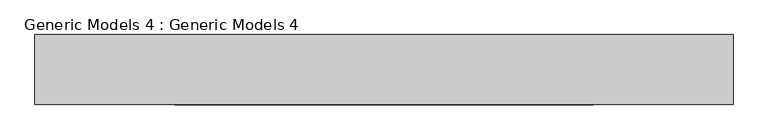
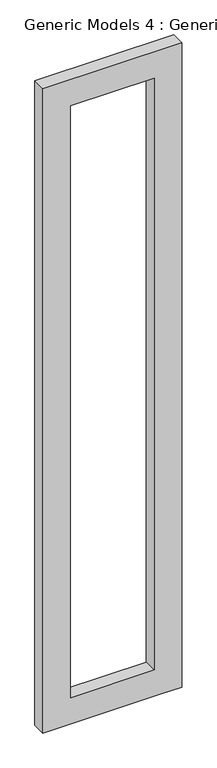
"""IFC4 building model written with IfcOpenShell, lengths in millimetres: proxy geometry, Generic Models 4 : Generic Models 4."""

from ifc_helpers import new_model, si_unit, frame, origin, place, context, project, spatial, polyline, outline, extrude, source, transform, mapped, element, save


def generic_models_4_generic_models_4_a39c55b3(model_context):
    return source(origin(), model_context, "Body", "SweptSolid", [
        extrude(outline(polyline([(7467.6, -14902.5371373), (7467.6, -16426.5371373), (0.0, -16426.5371373), (0.0, -15131.1371373), (0.0, -14902.5371373), (6426.2, -14902.5371373), (7467.6, -14902.5371373)]), holes=[polyline([(304.8, -16121.7371373), (7162.8, -16121.7371373), (7162.8, -15207.3371373), (304.8, -15207.3371373), (304.8, -16121.7371373)])]), frame((0.0, -3532.661407, 0.0), z_axis=(0.0, 1.0, 0.0), x_axis=(0.0, 0.0, 1.0)), (0.0, 0.0, 1.0), 152.4),
    ])


if __name__ == "__main__":
    model = new_model("IFC4")
    model_context = context("Model", 3, world=origin())
    ifc_project = project(units=[si_unit("LENGTHUNIT", "METRE", prefix="MILLI")], contexts=[model_context])
    site = spatial("IfcSite", under=ifc_project)
    building = spatial("IfcBuilding", under=site)
    placement = place(None, origin())
    generic_models_4_generic_models_4_shape = generic_models_4_generic_models_4_a39c55b3(model_context)
    element("IfcBuildingElementProxy", 1, Name="Generic Models 4 : Generic Models 4", ObjectType="Generic Models 4 : Generic Models 4", at=placement, inside=building, context=model_context, shape_type="MappedRepresentation", body=[
        mapped(generic_models_4_generic_models_4_shape, transform((0.0, 0.0, 0.0), x_axis=(1.0, 0.0, 0.0), y_axis=(0.0, 1.0, 0.0), z_axis=(0.0, 0.0, 1.0))),
    ])
    save(model, "model.ifc")
